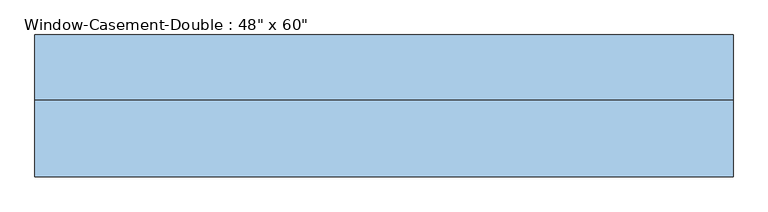
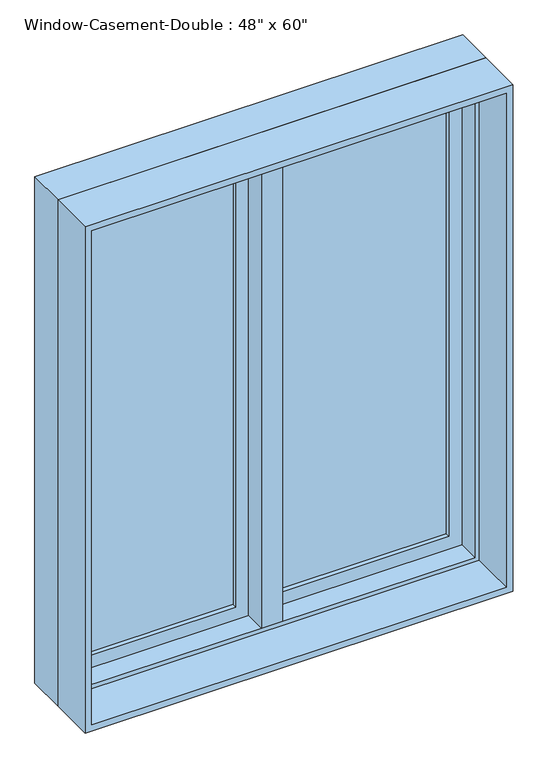
"""IFC4 building model written with IfcOpenShell, lengths in millimetres: window geometry."""

from ifc_helpers import new_model, si_unit, frame, origin, place, context, project, spatial, polyline, outline, extrude, faceted_brep, source, transform, mapped, element, save


def window_8377141f(model_context):
    return source(origin(), model_context, "Body", "SolidModel", [
        faceted_brep([(9.525, 133.35, 2425.7), (-9.525, 133.35, 2425.7), (-9.525, 82.55, 2425.7), (9.525, 82.55, 2425.7), (9.525, 133.35, 927.1), (9.525, 82.55, 927.1), (-9.525, 82.55, 927.1), (-9.525, 133.35, 927.1), (-9.525, 82.55, 946.15), (-9.525, 82.55, 2406.65), (-30.1625, 82.55, 946.15), (-30.1625, 82.55, 2406.65), (-30.1625, 19.05, 946.15), (-30.1625, 19.05, 2406.65), (30.1625, 19.05, 946.15), (30.1625, 19.05, 2406.65), (30.1625, 82.55, 946.15), (30.1625, 82.55, 2406.65), (9.525, 82.55, 946.15), (9.525, 82.55, 2406.65)], [[[0, 1, 2, 3]], [[4, 5, 6, 7]], [[1, 0, 4, 7]], [[2, 1, 7, 6, 8, 9]], [[9, 8, 10, 11]], [[11, 10, 12, 13]], [[13, 12, 14, 15]], [[15, 14, 16, 17]], [[17, 16, 18, 19]], [[0, 3, 19, 18, 5, 4]], [[18, 8, 6, 5]], [[9, 19, 3, 2]], [[8, 18, 16, 14, 12, 10]], [[19, 9, 11, 13, 15, 17]]]),
        extrude(outline(polyline([(-66.675, 114.3), (-66.675, 107.95), (-539.75, 107.95), (-539.75, 114.3), (-66.675, 114.3)])), frame((0.0, 0.0, 984.25), z_axis=(0.0, 0.0, 1.0), x_axis=(1.0, 0.0, 0.0)), (0.0, 0.0, 1.0), 1384.3),
        extrude(outline(polyline([(-539.75, 95.25), (-539.75, 101.6), (-66.675, 101.6), (-66.675, 95.25), (-539.75, 95.25)])), frame((0.0, 0.0, 984.25), z_axis=(0.0, 0.0, 1.0), x_axis=(1.0, 0.0, 0.0)), (0.0, 0.0, 1.0), 1384.3),
        extrude(outline(polyline([(539.75, 114.3), (539.75, 107.95), (66.675, 107.95), (66.675, 114.3), (539.75, 114.3)])), frame((0.0, 0.0, 984.25), z_axis=(0.0, 0.0, 1.0), x_axis=(1.0, 0.0, 0.0)), (0.0, 0.0, 1.0), 1384.3),
        extrude(outline(polyline([(66.675, 95.25), (66.675, 101.6), (539.75, 101.6), (539.75, 95.25), (66.675, 95.25)])), frame((0.0, 0.0, 984.25), z_axis=(0.0, 0.0, 1.0), x_axis=(1.0, 0.0, 0.0)), (0.0, 0.0, 1.0), 1384.3),
        extrude(outline(polyline([(2425.7, -596.9), (927.1, -596.9), (927.1, -9.525), (2425.7, -9.525), (2425.7, -596.9)]), holes=[polyline([(2368.55, -66.675), (984.25, -66.675), (984.25, -539.75), (2368.55, -539.75), (2368.55, -66.675)])]), frame((0.0, 82.55, 0.0), z_axis=(0.0, 1.0, 0.0), x_axis=(0.0, 0.0, 1.0)), (0.0, 0.0, 1.0), 44.45),
        extrude(outline(polyline([(927.1, 596.9), (2425.7, 596.9), (2425.7, 9.525), (927.1, 9.525), (927.1, 596.9)]), holes=[polyline([(984.25, 66.675), (2368.55, 66.675), (2368.55, 539.75), (984.25, 539.75), (984.25, 66.675)])]), frame((0.0, 82.55, 0.0), z_axis=(0.0, 1.0, 0.0), x_axis=(0.0, 0.0, 1.0)), (0.0, 0.0, 1.0), 44.45),
        extrude(outline(polyline([(2438.4, -609.6), (914.4, -609.6), (914.4, 609.6), (2438.4, 609.6), (2438.4, -609.6)]), holes=[polyline([(2419.35, 590.55), (933.45, 590.55), (933.45, -590.55), (2419.35, -590.55), (2419.35, 590.55)])]), frame((0.0, -114.3, 0.0), z_axis=(0.0, 1.0, 0.0), x_axis=(0.0, 0.0, 1.0)), (0.0, 0.0, 1.0), 133.35),
        faceted_brep([(577.85, 82.55, 2406.65), (577.85, 19.05, 2406.65), (-577.85, 19.05, 2406.65), (-577.85, 82.55, 2406.65), (596.9, 133.35, 2425.7), (596.9, 82.55, 2425.7), (-596.9, 82.55, 2425.7), (-596.9, 133.35, 2425.7), (609.6, 19.05, 2438.4), (609.6, 133.35, 2438.4), (-609.6, 133.35, 2438.4), (-609.6, 19.05, 2438.4), (-577.85, 19.05, 946.15), (-577.85, 82.55, 946.15), (-596.9, 82.55, 927.1), (-596.9, 133.35, 927.1), (-609.6, 133.35, 914.4), (-609.6, 19.05, 914.4), (577.85, 19.05, 946.15), (577.85, 82.55, 946.15), (596.9, 82.55, 927.1), (596.9, 133.35, 927.1), (609.6, 133.35, 914.4), (609.6, 19.05, 914.4)], [[[0, 1, 2, 3]], [[4, 5, 6, 7]], [[8, 9, 10, 11]], [[3, 2, 12, 13]], [[7, 6, 14, 15]], [[11, 10, 16, 17]], [[13, 12, 18, 19]], [[15, 14, 20, 21]], [[17, 16, 22, 23]], [[11, 17, 23, 8], [1, 18, 12, 2]], [[19, 18, 1, 0]], [[5, 20, 14, 6], [3, 13, 19, 0]], [[21, 20, 5, 4]], [[23, 22, 9, 8]], [[9, 22, 16, 10], [7, 15, 21, 4]]]),
    ])


if __name__ == "__main__":
    model = new_model("IFC4")
    model_context = context("Model", 3, world=origin())
    ifc_project = project(units=[si_unit("LENGTHUNIT", "METRE", prefix="MILLI")], contexts=[model_context])
    site = spatial("IfcSite", under=ifc_project)
    building = spatial("IfcBuilding", under=site)
    placement = place(None, origin())
    window_shape = window_8377141f(model_context)
    element("IfcWindow", 1, ObjectType="Window-Casement-Double : 48\" x 60\"", at=placement, inside=building, context=model_context, shape_type="MappedRepresentation", body=[
        mapped(window_shape, transform((0.0, 0.0, 0.0), x_axis=(1.0, 0.0, 0.0), y_axis=(0.0, 1.0, 0.0), z_axis=(0.0, 0.0, 1.0))),
    ])
    save(model, "model.ifc")

# Revit data of these elements
# Type "Window-Casement-Double : 48\" x 60\""
#   Type Mark = "16"
#   Fire Rating = "0.5h"
#   Assembly Code = "B2020100"
#   Analytic Construction = "Double glazing - domestic"
#   Frame Extension [instance default] = 0' - 0 1/4"
#   Window Inset [instance default] = 0' - 0"
#   Wall Thickness [instance default] = 0' - 6"
#   Interior Wall Closure [instance default] = 0' - 2 1/4"
#   Half Width = 2' - 0"
#   Visual Light Transmittance = 0.81
#   Thermal Resistance (R) = 1.8146 (h·ft²·°F)/BTU
#   Solar Heat Gain Coefficient = 0.76
#   Rough Width = 4' - 0 1/2"
#   Rough Height = 5' - 0 1/2"
#   Height = 5' - 0"
#   Heat Transfer Coefficient (U) = 0.5511 BTU/(h·ft²·°F)
#   Exterior Wall Closure [instance default] = 0' - 1 1/4"
#   Extension Jamb [instance default] = 0' - 2 1/4"
#   Default Sill Height = 3' - 0"
#   Width = 4' - 0"
#   Define Thermal Properties by = 0
#   Muntin Visibility = yes
#   Interior Trim Visibility [instance default] = yes
#   Exterior Trim Visibility [instance default] = yes
#   Extension Jamb Visibility [instance default] = yes
#   Interior Trim Material = Wood - Stained
#   Muntin Pattern = Muntin Pattern_2x2 : Muntin Pattern_2x2
#   Interior Trim = Trim-Window-Interior-Flat : Picture Frame
#   Interior Frame Material = Wood - Stained
#   Glass Panel Material = Glass
#   Exterior Trim Material = Clad - White
#   Exterior Trim = Trim-Window-Exterior-Flat : with Sill
#   Exterior Frame Material = Clad - White
#   Define Thermal Properties by = (empty or 0)
#   Wall Closure = (empty or 0)
# Element 1 (IfcWindow, "Window-Casement-Double : 48\" x 60\"")
#   Wall Thickness = 0' - 9"
#   Extension Jamb = 0' - 5 1/4"
#   Materials on its faces: "Wood - Stained", "Glass", "Clad - White"
# Materials
#   "Wood - Stained": class "Wood", colour RGB 173 132 96, transparency 0, Cost = 0
#   "Glass": class "Glass", colour RGB 245 245 243, transparency 1, Description = "Soda Lime Glass", Cost = 0
#   "Clad - White": class "Wood", colour RGB 245 245 243, transparency 0, Cost = 0
